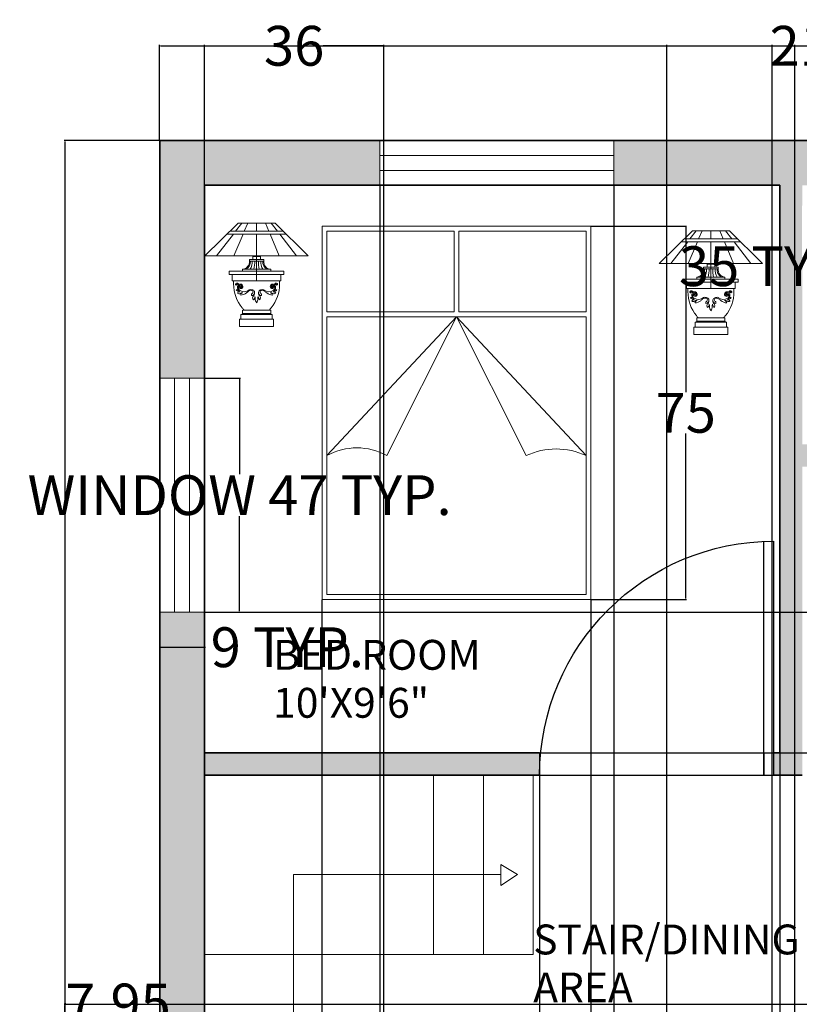
# Model space of a CAD drawing. Units: inches. Extents: x -24 to 368, y -370 to 58.
# Tile 7 of 9: x -24 to 133, y -140 to 58. Entities that reach past the tile are written whole.
import ezdxf

# ---------------------------------------------------------------- set-up
doc = ezdxf.new("R2010")
doc.units = ezdxf.units.IN
doc.header["$MEASUREMENT"] = 0
for name, color, linetype, lineweight in [('A-ANNO-DIMS', 2, 'Continuous', 18), ('A-AREA-IDEN', 7, 'Continuous', 18), ('A-FLOR-STRS', 7, 'Continuous', 18), ('A-WALL', 7, 'Continuous', 35), ('Furniture', 7, 'Continuous', 15)]:
    doc.layers.add(name, color=color, linetype=linetype, lineweight=lineweight)
for name, color, linetype, lineweight, true_color in [('A-DOOR', 40, 'Continuous', 25, 0xf8d731), ('A-GLAZ', 30, 'Continuous', 18, 0xf26722), ('A-WALL-PATT', 18, 'Continuous', 13, 0x000000)]:
    doc.layers.add(name, color=color, linetype=linetype, lineweight=lineweight, true_color=true_color)
doc.styles.get("Standard").update_dxf_attribs({"font": 'arial.ttf'})
doc.dimstyles.get("Standard").update_dxf_attribs({"dimtxt": 8, "dimasz": 0.18, "dimexe": 0.18, "dimexo": 0.0625, "dimgap": 0.09, "dimtad": 0, "dimtih": 1, "dimtoh": 1, "dimdec": 4, "dimzin": 0, "dimdsep": 46, "dimlunit": 3, "dimtxsty": 'Standard', "dimcen": 0.09, "dimclre": 5, "dimclrt": 6, "dimadec": 0, "dimazin": 0, "dimtfac": 1, "dimtdec": 4, "dimtofl": 0, "dimtmove": 0, "dimatfit": 3, "dimfxl": 1, "dimtolj": 1, "dimtzin": 0, "dimarcsym": 0})

# ---------------------------------------------------------------- blocks, each defined once
blk = doc.blocks.new('LAMP-BEDSIDE')
for p, q in [((6.65, 20.8), (0, 14.26)), ((6.17, 19.19), (7.42, 20.8)), ((6.65, 20.8), (14.09, 20.8)), ((8.59, 20.8), (7.91, 19.19)), ((10.37, 20.8), (10.37, 19.19)), ((12.15, 20.8), (12.83, 19.19)), ((14.57, 19.19), (13.31, 20.8)), ((14.09, 20.8), (20.74, 14.26)), ((2.33, 14.26), (5.71, 18.6)), ((4.42, 18.6), (16.32, 18.6)), ((5.01, 19.19), (15.72, 19.19)), ((7.66, 18.6), (5.82, 14.26)), ((10.37, 18.6), (10.37, 9.21)), ((13.08, 18.6), (14.92, 14.26)), ((18.41, 14.26), (15.02, 18.6)), ((0, 14.26), (20.74, 14.26)), ((9.6, 14.09), (11.14, 14.09)), ((9.6, 14.09), (9.6, 13.52)), ((11.14, 14.09), (11.14, 13.52)), ((8.92, 13.52), (11.81, 13.52)), ((8.92, 13.52), (8.92, 13.19)), ((8.92, 13.19), (11.81, 13.19)), ((11.81, 13.52), (11.81, 13.19)), ((4.88, 11.13), (4.88, 10.49)), ((4.88, 11.13), (15.86, 11.13)), ((4.88, 10.49), (15.86, 10.49)), ((5.48, 10.49), (5.48, 9.21)), ((7.53, 11.52), (13.2, 11.52)), ((7.53, 11.52), (7.53, 11.13)), ((13.2, 11.52), (13.2, 11.13)), ((15.26, 10.49), (15.26, 9.21)), ((15.86, 11.13), (15.86, 10.49)), ((5.48, 9.21), (15.26, 9.21)), ((5.76, 9.21), (5.76, 8.59)), ((14.98, 9.21), (14.98, 8.59)), ((7.24, 2.43), (10.37, 2.43)), ((7.24, 2.43), (7.24, 1.48)), ((7.53, 3.34), (10.37, 3.34)), ((7.53, 3.34), (7.53, 2.65)), ((7.53, 2.65), (10.37, 2.65)), ((13.2, 3.34), (10.37, 3.34)), ((13.2, 2.65), (10.37, 2.65)), ((13.5, 2.43), (10.37, 2.43)), ((13.2, 3.34), (13.2, 2.65)), ((13.5, 2.43), (13.5, 1.48)), ((6.96, 1.48), (6.96, 0)), ((6.96, 1.48), (7.24, 1.48)), ((6.96, 0), (10.37, 0)), ((7.24, 1.48), (10.37, 1.48)), ((13.5, 1.48), (10.37, 1.48)), ((13.77, 0), (10.37, 0)), ((13.77, 1.48), (13.5, 1.48)), ((13.77, 1.48), (13.77, 0))]:
    blk.add_line(p, q)
for centre, radius, start, end in [((7.4, 13.04), 1.53, 274.9221, 5.4044), ((7.51, 13), 1.63, 295.0919, 6.6681), ((6.74, 12.97), 2.77, 328.5732, 4.5839), ((4.28, 12.92), 5.72, 345.8511, 2.7031), ((16.46, 12.92), 5.72, 177.2969, 194.1489), ((14, 12.97), 2.77, 175.4161, 211.4268), ((13.22, 13), 1.63, 173.3319, 244.9081), ((13.33, 13.04), 1.53, 174.5956, 265.0779), ((13.2, 8.5), 7.44, 179.3119, 219.4824), ((6.29, 8.51), 0.158, 124.9924, 335.335), ((6.45, 8.39), 0.355, 11.1092, 135.0155), ((6.39, 8.42), 0.0502, 145.048, 23.2806), ((6.51, 8.39), 0.171, 352.7452, 159.4145), ((7.39, 7.88), 0.87, 145.6908, 234.6789), ((7.4, 7.83), 0.668, 137.9008, 234.3868), ((7.12, 8.07), 0.5, 320.8911, 130.3323), ((7.11, 7.94), 0.236, 29.1955, 234.854), ((7.14, 8.08), 0.309, 326.7711, 139.3622), ((7.2, 8), 0.128, 26.7504, 223.4128), ((13.61, 8.07), 0.5, 49.6677, 219.1089), ((7.54, 8.5), 7.44, 320.5176, 0.6881), ((13.6, 8.08), 0.309, 40.6378, 213.2289), ((13.63, 7.94), 0.236, 305.146, 150.8045), ((13.54, 8), 0.128, 316.5872, 153.2496), ((13.34, 7.83), 0.668, 305.6132, 42.0992), ((13.34, 7.88), 0.87, 305.3211, 34.3092), ((14.29, 8.39), 0.355, 44.9845, 168.8908), ((14.23, 8.39), 0.171, 20.5855, 187.2548), ((14.45, 8.51), 0.158, 204.665, 55.0076), ((14.35, 8.42), 0.0502, 156.7194, 34.952), ((6.44, 6.9), 0.527, 30.7639, 106.5031), ((6.66, 7.53), 0.391, 199.4301, 258.0626), ((6.99, 6.45), 0.534, 81.7725, 150.3347), ((6.86, 7.15), 0.552, 231.7834, 300.6647), ((6.55, 6.3), 0.85, 53.0509, 88.4488), ((7.24, 8), 0.363, 223.4201, 318.9658), ((7.88, 8.48), 1.48, 232.7522, 313.7075), ((7.25, 8.05), 0.203, 224.103, 315.897), ((7.49, 6.32), 0.495, 75.8737, 133.8842), ((7.68, 6.3), 0.502, 98.3136, 177.606), ((7.04, 8.37), 2.05, 274.0547, 309.0162), ((5.53, 10.82), 4.92, 304.6293, 311.2979), ((9.22, 6.66), 0.644, 58.6818, 132.9572), ((9.12, 6.87), 0.587, 71.5671, 111.734), ((9.36, 6.81), 0.621, 342.0461, 94.8157), ((9.69, 6.38), 0.339, 108.5318, 204.8769), ((9.33, 6.92), 0.689, 273.9841, 333.6418), ((9.32, 6.94), 0.352, 316.7375, 49.0095), ((10.14, 5.79), 0.564, 138.2432, 224.6957), ((9.31, 6.66), 0.643, 310.3655, 356.3809), ((8.93, 6.11), 1.09, 318.697, 356.3018), ((9.3, 5.7), 0.788, 353.0671, 25.9825), ((11.43, 5.7), 0.788, 154.0175, 186.9329), ((11.81, 6.11), 1.09, 183.6982, 221.303), ((11.38, 6.81), 0.621, 85.1843, 197.9539), ((11.41, 6.92), 0.689, 206.3582, 266.0159), ((11.43, 6.66), 0.643, 183.6191, 229.6345), ((10.59, 5.79), 0.564, 315.3043, 41.7568), ((11.41, 6.94), 0.352, 130.9905, 223.2625), ((11.05, 6.38), 0.339, 335.1231, 71.4682), ((11.52, 6.66), 0.644, 47.0428, 121.3182), ((11.62, 6.87), 0.587, 68.266, 108.4329), ((12.85, 8.48), 1.48, 226.2925, 307.2478), ((15.2, 10.82), 4.92, 228.7021, 235.3707), ((13.7, 8.37), 2.05, 230.9838, 265.9453), ((13.25, 6.32), 0.495, 46.1158, 104.1263), ((13.05, 6.3), 0.502, 2.394, 81.6864), ((13.5, 8), 0.363, 221.0342, 316.5799), ((13.48, 8.05), 0.203, 224.103, 315.897), ((13.87, 7.15), 0.552, 239.3353, 308.2166), ((14.18, 6.3), 0.85, 91.5512, 126.9491), ((13.75, 6.45), 0.534, 29.6653, 98.2275), ((14.3, 6.9), 0.527, 73.4969, 149.2361), ((14.08, 7.53), 0.391, 281.9374, 340.5699), ((12.16, 5.83), 2.09, 186.3334, 210.8958), ((8.58, 5.83), 2.09, 329.1042, 353.6666), ((7.29, 2.67), 0.245, 257.4164, 350.592), ((10.43, 6.05), 3.74, 217.4462, 226.2556), ((10.31, 6.05), 3.74, 313.7444, 322.5538), ((10.31, 6.05), 3.74, 313.7444, 322.5538), ((13.45, 2.67), 0.245, 189.408, 282.5836)]:
    blk.add_arc(centre, radius, start, end)
blk = doc.blocks.new('WINDOW-47-JAMB-DETAIL')
for p, q in [((0, 9), (47, 9)), ((0, 0), (0, 9)), ((0, 9), (0, 4.5)), ((47, 9), (47, 0)), ((0, 6), (47, 6)), ((0, 3), (47, 3)), ((47, 0), (0, 0))]:
    blk.add_line(p, q)
blk = doc.blocks.new('WINDOW-47')
for p, q in [((0, 47), (0, 0)), ((0, 47), (9, 47)), ((3, 47), (3, 0)), ((6, 47), (6, 0)), ((9, 0), (9, 47)), ((0, 0), (9, 0))]:
    blk.add_line(p, q)
blk = doc.blocks.new('DOOR-SINGLE-47')
for p, q in [((0, 0), (0, 47)), ((2, 0), (2, 47)), ((47, 0), (0, 0))]:
    blk.add_line(p, q)
blk.add_arc((0, 0), 47, 0, 90)
blk = doc.blocks.new('*D17')
at = {"layer": 'A-ANNO-DIMS', "color": 5, "lineweight": -2, "transparency": 16777216}
for p, q in [((13.22, -14.1), (20.39, -14.1)), ((13.22, -61.1), (20.39, -61.1))]:
    blk.add_line(p, q, dxfattribs=at)
at = {"layer": 'A-ANNO-DIMS', "color": 0, "lineweight": -2, "transparency": 16777216}
for p, q in [((20.21, -14.28), (20.21, -33.37)), ((20.21, -60.92), (20.21, -41.83))]:
    blk.add_line(p, q, dxfattribs=at)
at = {"layer": 'A-ANNO-DIMS', "color": 0, "transparency": 16777216}
for points in [[(20.18, -14.28), (20.24, -14.28), (20.21, -14.1)], [(20.18, -60.92), (20.24, -60.92), (20.21, -61.1)]]:
    blk.add_solid(points, dxfattribs=at)
at = {"layer": 'Defpoints', "color": 0, "transparency": 16777216}
for p in [(13.16, -14.1), (20.21, -14.1), (13.16, -61.1)]:
    blk.add_point(p, dxfattribs=at)
at = {"layer": 'A-ANNO-DIMS', "color": 6, "transparency": 16777216, "insert": (20.21, -37.6), "char_height": 8, "attachment_point": 5}
blk.add_mtext('\\A1;WINDOW 47 TYP.', dxfattribs=at)
blk = doc.blocks.new('*D18')
at = {"layer": 'A-ANNO-DIMS', "color": 5, "lineweight": -2, "transparency": 16777216}
for p, q in [((4.16, -61.16), (4.16, -68.33)), ((13.16, -61.16), (13.16, -68.33))]:
    blk.add_line(p, q, dxfattribs=at)
at = {"layer": 'A-ANNO-DIMS', "color": 0, "lineweight": -2, "transparency": 16777216}
for p, q in [((4.34, -68.15), (12.98, -68.15)), ((13.16, -68.15), (13.34, -68.15))]:
    blk.add_line(p, q, dxfattribs=at)
at = {"layer": 'A-ANNO-DIMS', "color": 0, "transparency": 16777216}
for points in [[(4.34, -68.12), (4.34, -68.18), (4.16, -68.15)], [(12.98, -68.12), (12.98, -68.18), (13.16, -68.15)]]:
    blk.add_solid(points, dxfattribs=at)
at = {"layer": 'Defpoints', "color": 0, "transparency": 16777216}
for p in [(4.16, -61.1), (13.16, -61.1), (13.16, -68.15)]:
    blk.add_point(p, dxfattribs=at)
at = {"layer": 'A-ANNO-DIMS', "color": 6, "transparency": 16777216, "insert": (29.79, -68.15), "char_height": 8, "attachment_point": 5}
blk.add_mtext('\\A1;9 TYP.', dxfattribs=at)
blk = doc.blocks.new('*D24')
at = {"layer": 'A-ANNO-DIMS', "color": 0, "lineweight": -2, "transparency": 16777216}
for p, q in [((146.57, 8.39), (146.39, 8.39)), ((181.39, 8.39), (146.75, 8.39))]:
    blk.add_line(p, q, dxfattribs=at)
at = {"layer": 'A-ANNO-DIMS', "color": 5, "lineweight": -2, "transparency": 16777216}
for p, q in [((146.57, 3.21), (146.57, 8.57)), ((181.57, 3.21), (181.57, 8.57))]:
    blk.add_line(p, q, dxfattribs=at)
at = {"layer": 'A-ANNO-DIMS', "color": 0, "transparency": 16777216}
for points in [[(146.75, 8.42), (146.75, 8.36), (146.57, 8.39)], [(181.39, 8.42), (181.39, 8.36), (181.57, 8.39)]]:
    blk.add_solid(points, dxfattribs=at)
at = {"layer": 'Defpoints', "color": 0, "transparency": 16777216}
for p in [(146.57, 8.39), (146.57, 3.14), (181.57, 3.14)]:
    blk.add_point(p, dxfattribs=at)
at = {"layer": 'A-ANNO-DIMS', "color": 6, "transparency": 16777216, "insert": (126.83, 8.39), "char_height": 8, "attachment_point": 5}
blk.add_mtext('\\A1;35 TYP.', dxfattribs=at)
blk = doc.blocks.new('*D25')
at = {"layer": 'A-ANNO-DIMS', "color": 5, "lineweight": -2, "transparency": 16777216}
for p, q in [((4.16, 33.71), (4.16, 52.85)), ((322.16, 33.71), (322.16, 52.85))]:
    blk.add_line(p, q, dxfattribs=at)
at = {"layer": 'A-ANNO-DIMS', "color": 0, "lineweight": -2, "transparency": 16777216}
for p, q in [((4.34, 52.67), (154.23, 52.67)), ((321.98, 52.67), (172.1, 52.67))]:
    blk.add_line(p, q, dxfattribs=at)
at = {"layer": 'A-ANNO-DIMS', "color": 0, "transparency": 16777216}
for points in [[(4.34, 52.7), (4.34, 52.64), (4.16, 52.67)], [(321.98, 52.7), (321.98, 52.64), (322.16, 52.67)]]:
    blk.add_solid(points, dxfattribs=at)
at = {"layer": 'Defpoints', "color": 0, "transparency": 16777216}
for p in [(322.16, 52.67), (4.16, 33.64), (322.16, 33.64)]:
    blk.add_point(p, dxfattribs=at)
at = {"layer": 'A-ANNO-DIMS', "color": 6, "transparency": 16777216, "insert": (163.16, 52.67), "char_height": 8, "attachment_point": 5}
blk.add_mtext('\\A1;318', dxfattribs=at)
blk = doc.blocks.new('*D26')
at = {"layer": 'A-ANNO-DIMS', "color": 5, "lineweight": -2, "transparency": 16777216}
for p, q in [((4.1, 33.64), (-15.03, 33.64)), ((4.1, -344.36), (-15.03, -344.36))]:
    blk.add_line(p, q, dxfattribs=at)
at = {"layer": 'A-ANNO-DIMS', "color": 0, "lineweight": -2, "transparency": 16777216}
for p, q in [((-14.85, 33.46), (-14.85, -151.18)), ((-14.85, -344.18), (-14.85, -159.53))]:
    blk.add_line(p, q, dxfattribs=at)
at = {"layer": 'A-ANNO-DIMS', "color": 0, "transparency": 16777216}
for points in [[(-14.88, 33.46), (-14.82, 33.46), (-14.85, 33.64)], [(-14.88, -344.18), (-14.82, -344.18), (-14.85, -344.36)]]:
    blk.add_solid(points, dxfattribs=at)
at = {"layer": 'Defpoints', "color": 0, "transparency": 16777216}
for p in [(-14.85, 33.64), (4.16, 33.64), (4.16, -344.36)]:
    blk.add_point(p, dxfattribs=at)
at = {"layer": 'A-ANNO-DIMS', "color": 6, "transparency": 16777216, "insert": (-14.85, -155.36), "char_height": 8, "attachment_point": 5}
blk.add_mtext('\\A1;378', dxfattribs=at)
blk = doc.blocks.new('*D40')
at = {"layer": 'A-ANNO-DIMS', "color": 5, "lineweight": -2, "transparency": 16777216}
for p, q in [((13.16, 24.58), (13.16, -363.55)), ((48.33, 24.58), (48.33, -363.55))]:
    blk.add_line(p, q, dxfattribs=at)
at = {"layer": 'A-ANNO-DIMS', "color": 0, "lineweight": -2, "transparency": 16777216}
for p, q in [((13.34, -363.37), (17.16, -363.37)), ((48.15, -363.37), (44.33, -363.37))]:
    blk.add_line(p, q, dxfattribs=at)
at = {"layer": 'A-ANNO-DIMS', "color": 0, "transparency": 16777216}
for points in [[(13.34, -363.34), (13.34, -363.4), (13.16, -363.37)], [(48.15, -363.34), (48.15, -363.4), (48.33, -363.37)]]:
    blk.add_solid(points, dxfattribs=at)
at = {"layer": 'Defpoints', "color": 0, "transparency": 16777216}
for p in [(13.16, 24.64), (48.33, 24.64), (48.33, -363.37)]:
    blk.add_point(p, dxfattribs=at)
at = {"layer": 'A-ANNO-DIMS', "color": 6, "transparency": 16777216, "insert": (30.75, -363.37), "char_height": 8, "attachment_point": 5}
blk.add_mtext('\\A1;35.17', dxfattribs=at)
blk = doc.blocks.new('*D41')
at = {"layer": 'A-ANNO-DIMS', "color": 5, "lineweight": -2, "transparency": 16777216}
for p, q in [((95.33, 24.58), (95.33, -363.55)), ((128.66, 24.58), (128.66, -363.55))]:
    blk.add_line(p, q, dxfattribs=at)
at = {"layer": 'A-ANNO-DIMS', "color": 0, "lineweight": -2, "transparency": 16777216}
for p, q in [((95.51, -363.37), (98.41, -363.37)), ((128.48, -363.37), (125.58, -363.37))]:
    blk.add_line(p, q, dxfattribs=at)
at = {"layer": 'A-ANNO-DIMS', "color": 0, "transparency": 16777216}
for points in [[(95.51, -363.34), (95.51, -363.4), (95.33, -363.37)], [(128.48, -363.34), (128.48, -363.4), (128.66, -363.37)]]:
    blk.add_solid(points, dxfattribs=at)
at = {"layer": 'Defpoints', "color": 0, "transparency": 16777216}
for p in [(95.33, 24.64), (128.66, 24.64), (128.66, -363.37)]:
    blk.add_point(p, dxfattribs=at)
at = {"layer": 'A-ANNO-DIMS', "color": 6, "transparency": 16777216, "insert": (112, -363.37), "char_height": 8, "attachment_point": 5}
blk.add_mtext('\\A1;33.33', dxfattribs=at)
blk = doc.blocks.new('*D44')
at = {"layer": 'A-ANNO-DIMS', "color": 5, "lineweight": -2, "transparency": 16777216}
for p, q in [((13.22, -61.1), (341.36, -61.1)), ((13.22, -89.36), (341.36, -89.36))]:
    blk.add_line(p, q, dxfattribs=at)
at = {"layer": 'A-ANNO-DIMS', "color": 0, "lineweight": -2, "transparency": 16777216}
for p, q in [((341.18, -61.28), (341.18, -71.05)), ((341.18, -89.18), (341.18, -79.4))]:
    blk.add_line(p, q, dxfattribs=at)
at = {"layer": 'A-ANNO-DIMS', "color": 0, "transparency": 16777216}
for points in [[(341.15, -61.28), (341.21, -61.28), (341.18, -61.1)], [(341.15, -89.18), (341.21, -89.18), (341.18, -89.36)]]:
    blk.add_solid(points, dxfattribs=at)
at = {"layer": 'Defpoints', "color": 0, "transparency": 16777216}
for p in [(13.16, -61.1), (341.18, -61.1), (13.16, -89.36)]:
    blk.add_point(p, dxfattribs=at)
at = {"layer": 'A-ANNO-DIMS', "color": 6, "transparency": 16777216, "insert": (341.18, -75.23), "char_height": 8, "attachment_point": 5}
blk.add_mtext('\\A1;28.26', dxfattribs=at)
blk = doc.blocks.new('*D47')
at = {"layer": 'A-ANNO-DIMS', "color": 5, "lineweight": -2, "transparency": 16777216}
for p, q in [((36.75, -58.62), (36.75, -363.55)), ((90.75, -58.62), (90.75, -363.55))]:
    blk.add_line(p, q, dxfattribs=at)
at = {"layer": 'A-ANNO-DIMS', "color": 0, "lineweight": -2, "transparency": 16777216}
for p, q in [((36.93, -363.37), (57.95, -363.37)), ((90.57, -363.37), (69.56, -363.37))]:
    blk.add_line(p, q, dxfattribs=at)
at = {"layer": 'A-ANNO-DIMS', "color": 0, "transparency": 16777216}
for points in [[(36.93, -363.34), (36.93, -363.4), (36.75, -363.37)], [(90.57, -363.34), (90.57, -363.4), (90.75, -363.37)]]:
    blk.add_solid(points, dxfattribs=at)
at = {"layer": 'Defpoints', "color": 0, "transparency": 16777216}
for p in [(36.75, -58.55), (90.75, -58.55), (90.75, -363.37)]:
    blk.add_point(p, dxfattribs=at)
at = {"layer": 'A-ANNO-DIMS', "color": 6, "transparency": 16777216, "insert": (63.75, -363.37), "char_height": 8, "attachment_point": 5}
blk.add_mtext('\\A1;54', dxfattribs=at)
blk = doc.blocks.new('*D48')
at = {"layer": 'A-ANNO-DIMS', "color": 5, "lineweight": -2, "transparency": 16777216}
for p, q in [((90.82, 16.45), (109.95, 16.45)), ((90.82, -58.55), (109.95, -58.55))]:
    blk.add_line(p, q, dxfattribs=at)
at = {"layer": 'A-ANNO-DIMS', "color": 0, "lineweight": -2, "transparency": 16777216}
for p, q in [((109.77, 16.27), (109.77, -16.9)), ((109.77, -58.37), (109.77, -25.21))]:
    blk.add_line(p, q, dxfattribs=at)
at = {"layer": 'A-ANNO-DIMS', "color": 0, "transparency": 16777216}
for points in [[(109.74, 16.27), (109.8, 16.27), (109.77, 16.45)], [(109.74, -58.37), (109.8, -58.37), (109.77, -58.55)]]:
    blk.add_solid(points, dxfattribs=at)
at = {"layer": 'Defpoints', "color": 0, "transparency": 16777216}
for p in [(90.75, 16.45), (90.75, -58.55), (109.77, -58.55)]:
    blk.add_point(p, dxfattribs=at)
at = {"layer": 'A-ANNO-DIMS', "color": 6, "transparency": 16777216, "insert": (109.77, -21.05), "char_height": 8, "attachment_point": 5}
blk.add_mtext('\\A1;75', dxfattribs=at)
blk = doc.blocks.new('*D49')
at = {"layer": 'A-ANNO-DIMS', "color": 5, "lineweight": -2, "transparency": 16777216}
for p, q in [((13.16, -149.79), (13.16, 52.85)), ((49.16, -149.79), (49.16, 52.85))]:
    blk.add_line(p, q, dxfattribs=at)
at = {"layer": 'A-ANNO-DIMS', "color": 0, "lineweight": -2, "transparency": 16777216}
for p, q in [((13.34, 52.67), (25.35, 52.67)), ((48.98, 52.67), (36.98, 52.67))]:
    blk.add_line(p, q, dxfattribs=at)
at = {"layer": 'A-ANNO-DIMS', "color": 0, "transparency": 16777216}
for points in [[(13.34, 52.7), (13.34, 52.64), (13.16, 52.67)], [(48.98, 52.7), (48.98, 52.64), (49.16, 52.67)]]:
    blk.add_solid(points, dxfattribs=at)
at = {"layer": 'Defpoints', "color": 0, "transparency": 16777216}
for p in [(49.16, 52.67), (13.16, -149.86), (49.16, -149.86)]:
    blk.add_point(p, dxfattribs=at)
at = {"layer": 'A-ANNO-DIMS', "color": 6, "transparency": 16777216, "insert": (31.16, 52.67), "char_height": 8, "attachment_point": 5}
blk.add_mtext('\\A1;36', dxfattribs=at)
blk = doc.blocks.new('*D53')
at = {"layer": 'A-ANNO-DIMS', "color": 5, "lineweight": -2, "transparency": 16777216}
for p, q in [((13.16, -89.42), (13.16, -363.55)), ((80.45, -89.42), (80.45, -363.55))]:
    blk.add_line(p, q, dxfattribs=at)
at = {"layer": 'A-ANNO-DIMS', "color": 0, "lineweight": -2, "transparency": 16777216}
for p, q in [((13.34, -363.37), (33.19, -363.37)), ((80.27, -363.37), (60.42, -363.37))]:
    blk.add_line(p, q, dxfattribs=at)
at = {"layer": 'A-ANNO-DIMS', "color": 0, "transparency": 16777216}
for points in [[(13.34, -363.34), (13.34, -363.4), (13.16, -363.37)], [(80.27, -363.34), (80.27, -363.4), (80.45, -363.37)]]:
    blk.add_solid(points, dxfattribs=at)
at = {"layer": 'Defpoints', "color": 0, "transparency": 16777216}
for p in [(13.16, -89.36), (80.45, -89.36), (80.45, -363.37)]:
    blk.add_point(p, dxfattribs=at)
at = {"layer": 'A-ANNO-DIMS', "color": 6, "transparency": 16777216, "insert": (46.81, -363.37), "char_height": 8, "attachment_point": 5}
blk.add_mtext('\\A1;67.29', dxfattribs=at)
blk = doc.blocks.new('*D55')
at = {"layer": 'A-ANNO-DIMS', "color": 5, "lineweight": -2, "transparency": 16777216}
for p, q in [((131.66, -152.29), (131.66, 52.85)), ((164.43, -152.29), (164.43, 52.85))]:
    blk.add_line(p, q, dxfattribs=at)
at = {"layer": 'A-ANNO-DIMS', "color": 0, "lineweight": -2, "transparency": 16777216}
for p, q in [((131.84, 52.67), (134.46, 52.67)), ((164.25, 52.67), (161.63, 52.67))]:
    blk.add_line(p, q, dxfattribs=at)
at = {"layer": 'A-ANNO-DIMS', "color": 0, "transparency": 16777216}
for points in [[(131.84, 52.7), (131.84, 52.64), (131.66, 52.67)], [(164.25, 52.7), (164.25, 52.64), (164.43, 52.67)]]:
    blk.add_solid(points, dxfattribs=at)
at = {"layer": 'Defpoints', "color": 0, "transparency": 16777216}
for p in [(164.43, 52.67), (131.66, -152.36), (164.43, -152.36)]:
    blk.add_point(p, dxfattribs=at)
at = {"layer": 'A-ANNO-DIMS', "color": 6, "transparency": 16777216, "insert": (148.05, 52.67), "char_height": 8, "attachment_point": 5}
blk.add_mtext('\\A1;32.77', dxfattribs=at)
blk = doc.blocks.new('*D59')
at = {"layer": 'A-ANNO-DIMS', "color": 5, "lineweight": -2, "transparency": 16777216}
for p, q in [((246.6, -139.91), (-15.03, -139.91)), ((246.6, -147.86), (-15.03, -147.86))]:
    blk.add_line(p, q, dxfattribs=at)
at = {"layer": 'A-ANNO-DIMS', "color": 0, "lineweight": -2, "transparency": 16777216}
for p, q in [((-14.85, -139.91), (-14.85, -139.73)), ((-14.85, -139.73), (-14.67, -139.73)), ((-14.85, -147.68), (-14.85, -140.09))]:
    blk.add_line(p, q, dxfattribs=at)
at = {"layer": 'A-ANNO-DIMS', "color": 0, "transparency": 16777216}
for points in [[(-14.88, -140.09), (-14.82, -140.09), (-14.85, -139.91)], [(-14.88, -147.68), (-14.82, -147.68), (-14.85, -147.86)]]:
    blk.add_solid(points, dxfattribs=at)
at = {"layer": 'Defpoints', "color": 0, "transparency": 16777216}
for p in [(-14.85, -139.91), (246.66, -139.91), (246.66, -147.86)]:
    blk.add_point(p, dxfattribs=at)
at = {"layer": 'A-ANNO-DIMS', "color": 6, "transparency": 16777216, "insert": (-4.2, -139.73), "char_height": 8, "attachment_point": 5}
blk.add_mtext('\\A1;7.95', dxfattribs=at)
blk = doc.blocks.new('*D65')
at = {"layer": 'A-ANNO-DIMS', "color": 5, "lineweight": -2, "transparency": 16777216}
for p, q in [((105.95, -335.29), (105.95, 52.85)), ((127.16, -335.29), (127.16, 52.85))]:
    blk.add_line(p, q, dxfattribs=at)
at = {"layer": 'A-ANNO-DIMS', "color": 0, "lineweight": -2, "transparency": 16777216}
for p, q in [((106.13, 52.67), (126.98, 52.67)), ((127.16, 52.67), (127.34, 52.67))]:
    blk.add_line(p, q, dxfattribs=at)
at = {"layer": 'A-ANNO-DIMS', "color": 0, "transparency": 16777216}
for points in [[(106.13, 52.7), (106.13, 52.64), (105.95, 52.67)], [(126.98, 52.7), (126.98, 52.64), (127.16, 52.67)]]:
    blk.add_solid(points, dxfattribs=at)
at = {"layer": 'Defpoints', "color": 0, "transparency": 16777216}
for p in [(127.16, 52.67), (105.95, -335.36), (127.16, -335.36)]:
    blk.add_point(p, dxfattribs=at)
at = {"layer": 'A-ANNO-DIMS', "color": 6, "transparency": 16777216, "insert": (140.23, 52.67), "char_height": 8, "attachment_point": 5}
blk.add_mtext('\\A1;21.21', dxfattribs=at)

msp = doc.modelspace()

# ---------------------------------------------------------------- hatches: boundary and pattern name
at = {"layer": 'A-WALL-PATT'}
h = msp.add_hatch(color=256, dxfattribs=at)
h.dxf.hatch_style = 1
h.paths.add_polyline_path([(13.1621, -93.8573), (80.4499, -93.8573), (80.4499, -89.3573), (13.1621, -89.3573), (13.1621, -61.0987), (4.1621, -61.0987), (4.1621, -149.8573), (13.1621, -149.8573)])
h.paths.add_polyline_path([(146.5668, -27.3573), (133.1621, -27.3573), (133.1621, 10.3323), (133.1272, 10.3313), (133.1621, 24.6427), (139.8141, 24.6427), (139.8141, 33.6427), (95.3329, 33.6427), (95.3329, 24.6427), (128.6621, 24.6427), (128.6621, -89.3573), (127.4499, -89.3573), (127.4499, -93.8573), (133.1621, -93.8573), (133.1621, -31.8573), (146.5668, -31.8573)])
h.paths.add_polyline_path([(197.6621, 24.6427), (236.2134, 24.6427), (236.2134, 33.6427), (169.8141, 33.6427), (169.8141, 24.6427), (193.1621, 24.6427), (193.1621, -27.3573), (181.5668, -27.3573), (181.5668, -31.8573), (193.1621, -31.8573), (193.1621, -95.8573), (199.2127, -95.8573), (199.2127, -91.3573), (197.6621, -91.3573)])
h.paths.add_polyline_path([(322.1621, -52.531), (313.1621, -52.531), (313.1621, -91.3573), (246.2127, -91.3573), (246.2127, -95.8573), (246.6621, -95.8573), (246.6621, -104.9077), (251.1621, -104.9077), (251.1621, -95.8573), (313.1621, -95.8573), (313.1621, -105.6922), (317.6621, -105.6922), (322.1621, -105.6922)])
h.paths.add_polyline_path([(322.1621, -135.6922), (313.1621, -135.6922), (313.1621, -147.8573), (251.1621, -147.8573), (251.1621, -139.9077), (246.6621, -139.9077), (246.6621, -147.8573), (199.43, -147.8573), (199.43, -152.3573), (313.1621, -152.3573), (313.1621, -194.6142), (317.6621, -194.6142), (322.1621, -194.6142)])
h.paths.add_polyline_path([(322.1621, -241.6142), (313.1621, -241.6142), (313.1621, -275.3573), (287.3912, -275.3573), (287.3912, -279.8573), (313.1621, -279.8573), (313.1621, -335.3573), (298.077, -335.3573), (298.077, -344.3573), (322.1621, -344.3573)])
h.paths.add_polyline_path([(263.077, -335.3573), (241.1621, -335.3573), (241.1621, -279.8573), (252.3912, -279.8573), (252.3912, -275.3573), (236.6621, -275.3573), (236.6621, -298.8573), (234.5689, -298.8573), (234.5689, -303.3573), (236.6621, -303.3573), (236.6621, -344.3573), (263.077, -344.3573), (263.077, -339.8573)])
h.paths.add_polyline_path([(175.5689, -298.8573), (131.6621, -298.8573), (131.6621, -152.3573), (164.43, -152.3573), (164.43, -147.8573), (127.1621, -147.8573), (127.1621, -232.8573), (117.1621, -232.8573), (117.1621, -237.3573), (127.1621, -237.3573), (127.1621, -335.3573), (84.4055, -335.3573), (84.4055, -344.3573), (131.6621, -344.3573), (131.6621, -303.3573), (175.5689, -303.3573)])
h.paths.add_polyline_path([(70.1621, -232.8573), (13.1621, -232.8573), (13.1621, -196.8573), (4.1621, -196.8573), (4.1621, -257.9061), (13.1621, -257.9061), (13.1621, -237.3573), (70.1621, -237.3573)])
h.paths.add_polyline_path([(13.1621, -304.9061), (4.1621, -304.9061), (4.1621, -344.3573), (37.4055, -344.3573), (37.4055, -335.3573), (13.1621, -335.3573)])
h.paths.add_polyline_path([(322.1621, 33.6427), (283.2134, 33.6427), (283.2134, 24.6427), (313.1621, 24.6427), (313.1621, 11.9273), (313.4656, 11.629), (313.1621, 11.629), (313.1621, -5.531), (322.1621, -5.531)])
h.paths.add_polyline_path([(48.3329, 33.6427), (4.1621, 33.6427), (4.1621, -14.0987), (13.1621, -14.0987), (13.1621, 24.6427), (48.3329, 24.6427)])

# ---------------------------------------------------------------- linework, layer by layer
at = {"layer": 'A-DOOR'}
for p, q in [((80.4499, -89.3573), (80.4499, -93.8573)), ((125.4499, -89.3573), (125.4499, -93.8573))]:
    msp.add_line(p, q, dxfattribs=at)
at = {"layer": 'A-FLOR-STRS'}
for p, q in [((49.1621, -232.8573), (49.1621, -93.8573)), ((59.1621, -129.8573), (59.1621, -93.8573)), ((69.1621, -129.8573), (69.1621, -93.8573)), ((79.1621, -129.8573), (79.1621, -93.8573)), ((72.6401, -113.8048), (72.6401, -111.8048)), ((72.6401, -111.8048), (75.9936, -113.8048)), ((31.0603, -214.8573), (31.0603, -113.8048)), ((31.0603, -113.8048), (72.6401, -113.8048)), ((75.9936, -113.8048), (72.6401, -116.0308)), ((72.6401, -116.0308), (72.6401, -113.8048)), ((13.1621, -129.8573), (79.1621, -129.8573)), ((13.1621, -139.8573), (49.1621, -139.8573))]:
    msp.add_line(p, q, dxfattribs=at)
at = {"layer": 'A-WALL'}
for p, q in [((4.1621, -344.3573), (4.1621, 33.6427)), ((4.1621, 33.6427), (322.1621, 33.6427)), ((13.1621, 24.6427), (128.6621, 24.6427)), ((13.1621, -89.3573), (13.1621, 24.6427)), ((128.6621, -89.3573), (128.6621, 24.6427)), ((13.1621, -89.3573), (80.4499, -89.3573)), ((127.4499, -89.3573), (128.6621, -89.3573)), ((13.1621, -93.8573), (80.4499, -93.8573)), ((13.1621, -232.8573), (13.1621, -93.8573)), ((127.4499, -93.8573), (133.1621, -93.8573))]:
    msp.add_line(p, q, dxfattribs=at)
at = {"layer": 'Furniture'}
for p, q in [((63.2545, -0.7542), (63.2545, 15.4453)), ((64.2545, -0.7542), (64.2545, 15.4453)), ((37.7545, -0.7542), (63.2545, -0.7542)), ((37.7545, -1.7542), (89.7545, -1.7542)), ((63.7545, -1.7542), (37.7545, -29.6544)), ((49.7545, -29.6544), (63.7545, -1.7542)), ((63.7545, -1.7542), (89.7545, -29.6544)), ((77.7545, -29.6544), (63.7545, -1.7542)), ((64.2545, -0.7542), (89.7545, -0.7542))]:
    msp.add_line(p, q, dxfattribs=at)
msp.add_lwpolyline([(90.7545, 16.4453), (90.7545, -58.5547), (36.7545, -58.5547), (36.7545, 16.4453)], close=True, dxfattribs=at)
for points in [[(37.7545, -0.7542), (37.7545, 15.4453), (63.2545, 15.4453)], [(64.2545, 15.4453), (89.7545, 15.4453), (89.7545, -0.7542)], [(89.7545, -1.7542), (89.7545, -57.5547), (37.7545, -57.5547), (37.7545, -1.7542)]]:
    msp.add_lwpolyline(points, dxfattribs=at)
for centre, radius, start, end in [((43.7545, -40.4449), 12.3464, 60.923935, 119.076065), ((83.7545, -42.3825), 14.0713, 64.760772, 115.239228)]:
    msp.add_arc(centre, radius, start, end, dxfattribs=at)

# ---------------------------------------------------------------- block references
at = {"layer": 'A-DOOR', "extrusion": (0, 0, -1), "zscale": -1}
msp.add_blockref('DOOR-SINGLE-47', (-127.4496, -93.857), dxfattribs=at)
at = {"layer": 'A-GLAZ'}
for name, p in [('WINDOW-47-JAMB-DETAIL', (48.3325, 24.643)), ('WINDOW-47', (4.162, -61.0986))]:
    msp.add_blockref(name, p, dxfattribs=at)
at = {"layer": 'Furniture'}
for p in [(13.247, -3.751), (104.4562, -5.3093)]:
    msp.add_blockref('LAMP-BEDSIDE', p, dxfattribs=at)

# ---------------------------------------------------------------- texts
at = {"layer": 'A-AREA-IDEN'}
for s, p in [('BED ROOM', (26.9486, -72.6766)), ('10\'X9\'6"', (26.9486, -82.3151)), ('STAIR/DINING', (79.1621, -129.8573)), ('AREA', (79.1621, -139.4958))]:
    msp.add_text(s, height=6, dxfattribs=at).set_placement(p)

# ---------------------------------------------------------------- dimensions: what is measured, and where the dimension line sits
at = {"layer": 'A-ANNO-DIMS'}
for base, p1, p2, override, picture, middle in [((322.1621, 52.6658), (4.1621, 33.6427), (322.1621, 33.6427), {"dimdec": 0, "dimlfac": 1, "dimrnd": 0, "dimzin": 0, "dimdsep": 46, "dimlunit": 2}, '*D25', (163.1621, 52.6658)), ((49.1621, 52.6658), (13.1621, -149.8573), (49.1621, -149.8573), {"dimdec": 0, "dimlfac": 1, "dimrnd": 0, "dimzin": 0, "dimdsep": 46, "dimlunit": 2}, '*D49', (31.1621, 52.6658)), ((127.1621, 52.6658), (105.953, -335.3573), (127.1621, -335.3573), {"dimdec": 2, "dimlfac": 1, "dimrnd": 0, "dimzin": 0, "dimdsep": 46, "dimlunit": 2}, '*D65', (140.2261, 52.6658)), ((164.43, 52.6658), (131.6621, -152.3573), (164.43, -152.3573), {"dimdec": 2, "dimlfac": 1, "dimrnd": 0, "dimzin": 0, "dimdsep": 46, "dimlunit": 2}, '*D55', (148.046, 52.6658)), ((48.3329, -363.3723), (13.1621, 24.6427), (48.3329, 24.6427), {"dimdec": 2, "dimlfac": 1, "dimrnd": 0, "dimzin": 0, "dimdsep": 46, "dimlunit": 2}, '*D40', (30.7475, -363.3723)), ((128.6621, -363.3723), (95.3329, 24.6427), (128.6621, 24.6427), {"dimdec": 2, "dimlfac": 1, "dimrnd": 0, "dimzin": 0, "dimdsep": 46, "dimlunit": 2}, '*D41', (111.9975, -363.3723)), ((90.7545, -363.3723), (36.7545, -58.5547), (90.7545, -58.5547), {"dimdec": 0, "dimlfac": 1, "dimrnd": 0, "dimzin": 0, "dimdsep": 46, "dimlunit": 2}, '*D47', (63.7545, -363.3723)), ((80.4499, -363.3723), (13.1621, -89.3573), (80.4499, -89.3573), {"dimdec": 2, "dimlfac": 1, "dimrnd": 0, "dimzin": 0, "dimdsep": 46, "dimlunit": 2}, '*D53', (46.806, -363.3723))]:
    dim = msp.add_linear_dim(base=base, p1=p1, p2=p2, dimstyle='Standard', override=override, dxfattribs=at)
    dim.commit()
    dim.dimension.update_dxf_attribs({"geometry": picture, "text_midpoint": middle})
for base, p1, p2, angle, override, picture, middle in [((-14.8529, 33.6427), (4.1621, -344.3573), (4.1621, 33.6427), 90, {"dimdec": 0, "dimlfac": 1, "dimrnd": 0, "dimzin": 0, "dimdsep": 46, "dimlunit": 2}, '*D26', (-14.8529, -155.3573)), ((109.7695, -58.5547), (90.7545, 16.4453), (90.7545, -58.5547), 270, {"dimdec": 0, "dimlfac": 1, "dimrnd": 0, "dimzin": 0, "dimdsep": 46, "dimlunit": 2}, '*D48', (109.7695, -21.0547)), ((341.1771, -61.0987), (13.1621, -89.3573), (13.1621, -61.0987), 90, {"dimdec": 2, "dimlfac": 1, "dimrnd": 0, "dimzin": 0, "dimdsep": 46, "dimlunit": 2}, '*D44', (341.1771, -75.228)), ((-14.8529, -139.9077), (246.6621, -147.8573), (246.6621, -139.9077), 90, {"dimdec": 2, "dimlfac": 1, "dimrnd": 0, "dimzin": 0, "dimdsep": 46, "dimlunit": 2}, '*D59', (-4.1955, -139.7277))]:
    dim = msp.add_linear_dim(base=base, p1=p1, p2=p2, angle=angle, dimstyle='Standard', override=override, dxfattribs=at)
    dim.commit()
    dim.dimension.update_dxf_attribs({"geometry": picture, "text_midpoint": middle})
for base, p1, p2, angle, text, picture, middle in [((146.5668, 8.3927), (181.5668, 3.1427), (146.5668, 3.1427), 180, '<> TYP.', '*D24', (126.8289, 8.3927)), ((20.2121, -14.0987), (13.1621, -61.0987), (13.1621, -14.0987), 90, 'WINDOW <> TYP.', '*D17', (20.2121, -37.5987))]:
    dim = msp.add_linear_dim(base=base, p1=p1, p2=p2, angle=angle, text=text, dimstyle='Standard', override={"dimdec": 0, "dimlfac": 1, "dimrnd": 0, "dimzin": 0, "dimdsep": 46, "dimlunit": 2}, dxfattribs=at)
    dim.commit()
    dim.dimension.update_dxf_attribs({"geometry": picture, "text_midpoint": middle})
dim = msp.add_linear_dim(base=(13.1621, -68.1487), p1=(4.1621, -61.0987), p2=(13.1621, -61.0987), text='<> TYP.', dimstyle='Standard', override={"dimdec": 0, "dimlfac": 1, "dimrnd": 0, "dimzin": 0, "dimdsep": 46, "dimlunit": 2}, dxfattribs=at)
dim.commit()
dim.dimension.update_dxf_attribs({"geometry": '*D18', "text_midpoint": (29.795, -68.1487)})

doc.saveas('drawing.dxf')
